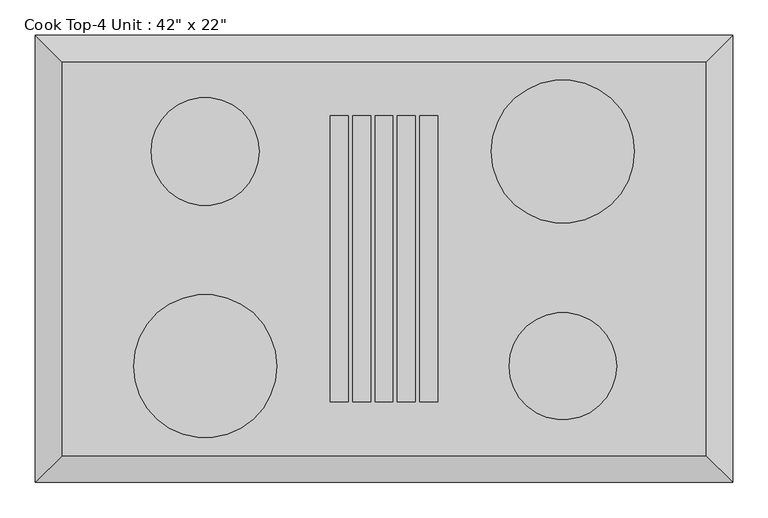
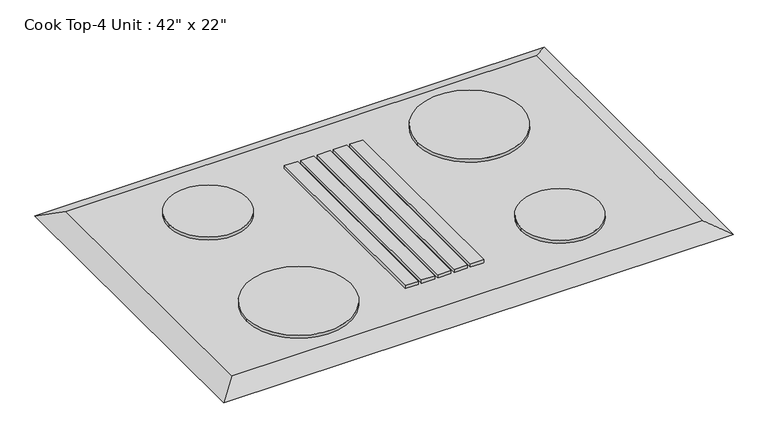
"""IFC4 building model written with IfcOpenShell, lengths in millimetres: proxy geometry."""

from ifc_helpers import new_model, si_unit, point, frame, frame_2d, origin, place, context, project, spatial, polyline, circle_curve, trimmed, segment, composite_curve, outline, extrude, faceted_brep, source, transform, mapped, element, save


def proxy_a120491f(model_context):
    return source(origin(), model_context, "Body", "SolidModel", [
        extrude(outline(composite_curve([segment(trimmed(circle_curve(frame_2d((-254.0, 152.4)), 76.5869489), [point((-177.4130511, 152.4))], [point((-330.5869489, 152.4))], False, "CARTESIAN"), True, "CONTINUOUS"), segment(trimmed(circle_curve(frame_2d((-254.0, 152.4)), 76.5869489), [point((-330.5869489, 152.4))], [point((-177.4130511, 152.4))], False, "CARTESIAN"), True, "CONTINUOUS")], self_intersect=False)), frame((0.0, 0.0, 806.45), z_axis=(0.0, 0.0, 1.0), x_axis=(1.0, 0.0, 0.0)), (0.0, 0.0, 1.0), 6.35),
        extrude(outline(composite_curve([segment(trimmed(circle_curve(frame_2d((254.0, 152.4)), 101.6), [point((355.6, 152.4))], [point((152.4, 152.4))], False, "CARTESIAN"), True, "CONTINUOUS"), segment(trimmed(circle_curve(frame_2d((254.0, 152.4)), 101.6), [point((152.4, 152.4))], [point((355.6, 152.4))], False, "CARTESIAN"), True, "CONTINUOUS")], self_intersect=False)), frame((0.0, 0.0, 806.45), z_axis=(0.0, 0.0, 1.0), x_axis=(1.0, 0.0, 0.0)), (0.0, 0.0, 1.0), 6.35),
        extrude(outline(composite_curve([segment(trimmed(circle_curve(frame_2d((254.0, -152.4)), 76.2), [point((330.2, -152.4))], [point((177.8, -152.4))], False, "CARTESIAN"), True, "CONTINUOUS"), segment(trimmed(circle_curve(frame_2d((254.0, -152.4)), 76.2), [point((177.8, -152.4))], [point((330.2, -152.4))], False, "CARTESIAN"), True, "CONTINUOUS")], self_intersect=False)), frame((0.0, 0.0, 806.45), z_axis=(0.0, 0.0, 1.0), x_axis=(1.0, 0.0, 0.0)), (0.0, 0.0, 1.0), 6.35),
        extrude(outline(polyline([(-50.8, 203.2), (-50.8, -203.2), (-76.2, -203.2), (-76.2, 203.2), (-50.8, 203.2)])), frame((0.0, 0.0, 806.45), z_axis=(0.0, 0.0, 1.0), x_axis=(1.0, 0.0, 0.0)), (0.0, 0.0, 1.0), 6.35),
        extrude(outline(polyline([(-19.05, 203.2), (-19.05, -203.2), (-44.45, -203.2), (-44.45, 203.2), (-19.05, 203.2)])), frame((0.0, 0.0, 806.45), z_axis=(0.0, 0.0, 1.0), x_axis=(1.0, 0.0, 0.0)), (0.0, 0.0, 1.0), 6.35),
        extrude(outline(polyline([(12.7, 203.2), (12.7, -203.2), (-12.7, -203.2), (-12.7, 203.2), (12.7, 203.2)])), frame((0.0, 0.0, 806.45), z_axis=(0.0, 0.0, 1.0), x_axis=(1.0, 0.0, 0.0)), (0.0, 0.0, 1.0), 6.35),
        extrude(outline(polyline([(44.45, 203.2), (44.45, -203.2), (19.05, -203.2), (19.05, 203.2), (44.45, 203.2)])), frame((0.0, 0.0, 806.45), z_axis=(0.0, 0.0, 1.0), x_axis=(1.0, 0.0, 0.0)), (0.0, 0.0, 1.0), 6.35),
        extrude(outline(polyline([(76.2, 203.2), (76.2, -203.2), (50.8, -203.2), (50.8, 203.2), (76.2, 203.2)])), frame((0.0, 0.0, 806.45), z_axis=(0.0, 0.0, 1.0), x_axis=(1.0, 0.0, 0.0)), (0.0, 0.0, 1.0), 6.35),
        faceted_brep([(457.2, 279.4, 806.45), (-457.2, 279.4, 806.45), (-457.2, -279.4, 806.45), (457.2, -279.4, 806.45), (495.3, 317.5, 787.4), (495.3, -317.5, 787.4), (-495.3, -317.5, 787.4), (-495.3, 317.5, 787.4)], [[[0, 1, 2, 3]], [[4, 5, 6, 7]], [[4, 7, 1, 0]], [[7, 6, 2, 1]], [[6, 5, 3, 2]], [[5, 4, 0, 3]]]),
        extrude(outline(composite_curve([segment(trimmed(circle_curve(frame_2d((-254.0, -152.4)), 101.6), [point((-152.4, -152.4))], [point((-355.6, -152.4))], False, "CARTESIAN"), True, "CONTINUOUS"), segment(trimmed(circle_curve(frame_2d((-254.0, -152.4)), 101.6), [point((-355.6, -152.4))], [point((-152.4, -152.4))], False, "CARTESIAN"), True, "CONTINUOUS")], self_intersect=False)), frame((0.0, 0.0, 806.45), z_axis=(0.0, 0.0, 1.0), x_axis=(1.0, 0.0, 0.0)), (0.0, 0.0, 1.0), 6.35),
    ])


if __name__ == "__main__":
    model = new_model("IFC4")
    model_context = context("Model", 3, world=origin())
    ifc_project = project(units=[si_unit("LENGTHUNIT", "METRE", prefix="MILLI")], contexts=[model_context])
    site = spatial("IfcSite", under=ifc_project)
    building = spatial("IfcBuilding", under=site)
    placement = place(None, origin())
    proxy_shape = proxy_a120491f(model_context)
    element("IfcBuildingElementProxy", 1, Name="Cook Top-4 Unit : 42\" x 22\"", ObjectType="Cook Top-4 Unit : 42\" x 22\"", at=placement, inside=building, context=model_context, shape_type="MappedRepresentation", body=[
        mapped(proxy_shape, transform((0.0, 0.0, 0.0), x_axis=(1.0, 0.0, 0.0), y_axis=(0.0, 1.0, 0.0), z_axis=(0.0, 0.0, 1.0))),
    ])
    save(model, "model.ifc")

# Revit data of these elements
# Type "Cook Top-4 Unit : 42\" x 22\""
#   Assembly Code = "E1090400"
#   Depth = 1' - 10"
#   Width = 3' - 0"
#   Burner Material = Steel, Chrome Plated
#   Cooktop Material = Steel, Polished
#   Default Elevation = 0
# Element 1 (IfcBuildingElementProxy, "Cook Top-4 Unit : 42\" x 22\"")
#   Materials on its faces: "Steel, Chrome Plated", "Steel, Polished"
# Materials
#   "Steel, Chrome Plated": class "Metal", colour RGB 17 17 17, transparency 0, Description = "Chromiuim plated steel", Cost = 0
#   "Steel, Polished": class "Metal", colour RGB 192 192 192, transparency 0, Description = "Polished steel", Cost = 0
